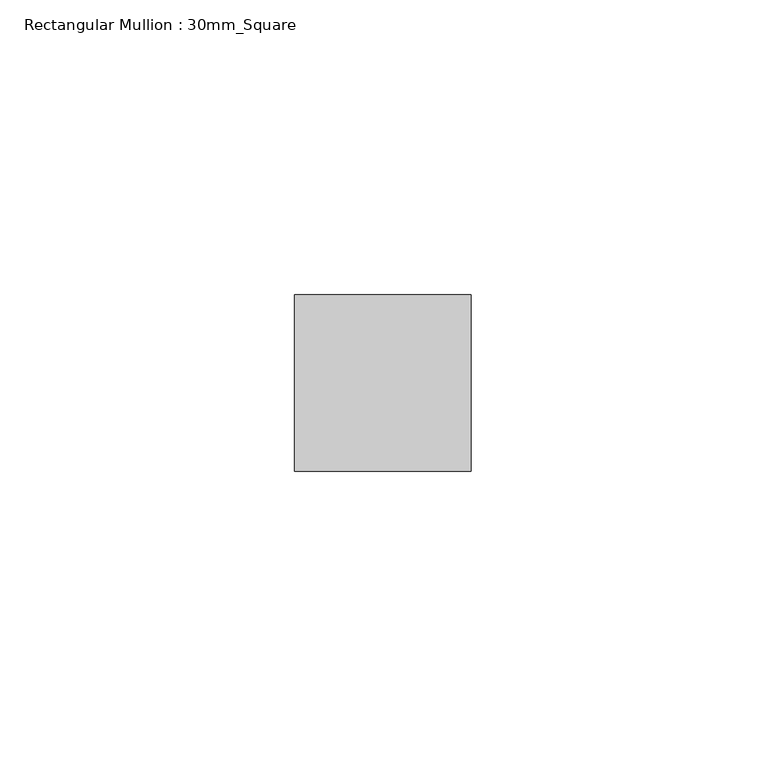
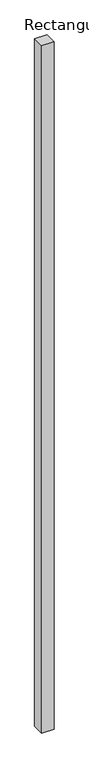
"""IFC4 building model written with IfcOpenShell, lengths in millimetres: member geometry, Rectangular Mullion : 30mm_Square."""

from ifc_helpers import new_model, si_unit, frame, origin, place, context, project, spatial, polyline, outline, extrude, source, transform, mapped, element, save


def rectangular_mullion_30mm_square_5f4e9219(model_context):
    return source(origin(), model_context, "Body", "SweptSolid", [
        extrude(outline(polyline([(0.0, 15.0), (0.0, -15.0), (-30.0, -15.0), (-30.0, 15.0), (0.0, 15.0)])), frame((0.0, 0.0, -1782.5999997), z_axis=(0.0, 0.0, 1.0), x_axis=(1.0, 0.0, 0.0)), (0.0, 0.0, 1.0), 1782.5999997),
    ])


if __name__ == "__main__":
    model = new_model("IFC4")
    model_context = context("Model", 3, world=origin())
    ifc_project = project(units=[si_unit("LENGTHUNIT", "METRE", prefix="MILLI")], contexts=[model_context])
    site = spatial("IfcSite", under=ifc_project)
    building = spatial("IfcBuilding", under=site)
    placement = place(None, origin())
    rectangular_mullion_30mm_square_shape = rectangular_mullion_30mm_square_5f4e9219(model_context)
    element("IfcMember", 1, ObjectType="Rectangular Mullion : 30mm_Square", at=placement, inside=building, context=model_context, shape_type="MappedRepresentation", body=[
        mapped(rectangular_mullion_30mm_square_shape, transform((0.0, 0.0, 0.0), x_axis=(1.0, 0.0, 0.0), y_axis=(0.0, 1.0, 0.0), z_axis=(0.0, 0.0, 1.0))),
    ])
    save(model, "model.ifc")

# Revit data of these elements
# Type "Rectangular Mullion : 30mm_Square"
#   Keynote = "H11"
#   built-in parameter 1007304 = 0.0984252 (stored number, unit not read)
#   built-in parameter 1007301 = 0.0492126 (stored number, unit not read)
#   built-in parameter 1007300 = 0.0492126 (stored number, unit not read)
# Element 1 (IfcMember, "Rectangular Mullion : 30mm_Square")
#   Materials on its faces: "Aluminium"
# Materials
#   "Aluminium": class "Metal", colour RGB 247 247 247, transparency 0, Description = "Aluminium 6061", Cost = 0
